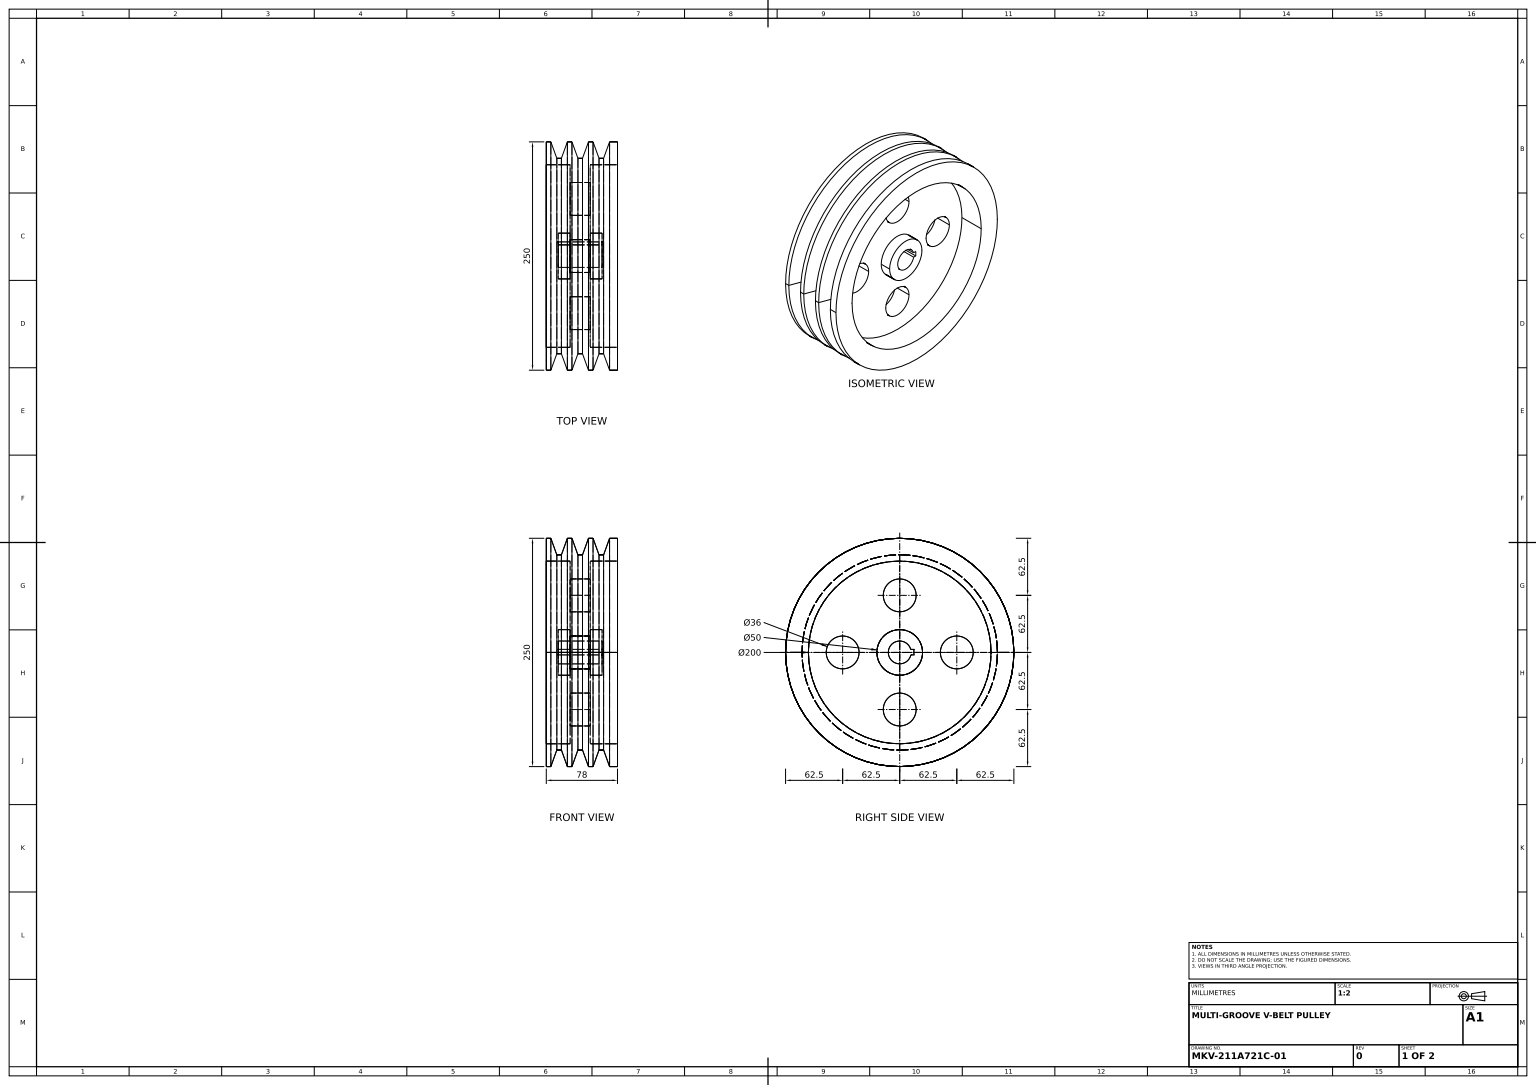
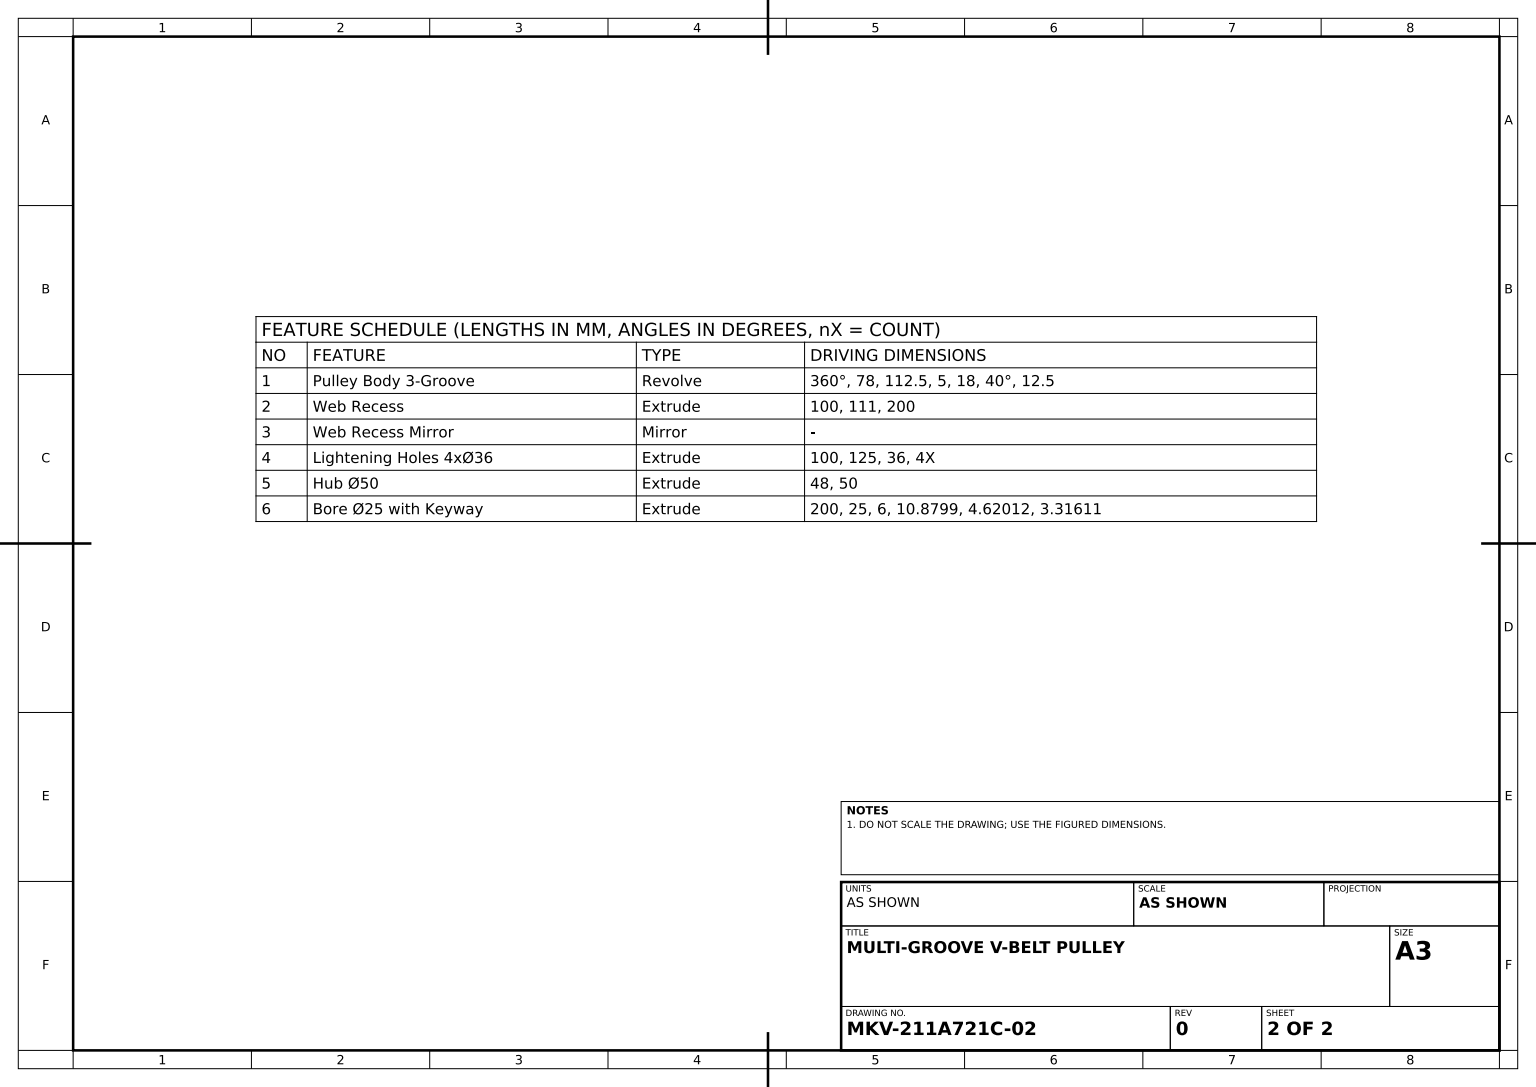
from build123d import *

# Parameters (mm, degrees)
WEB_START                    = 111
WEB_RECESS_SKETCH_R          = 100
WEB_RECESS_DEPTH             = 100
LIGHTENING_HOLES_SKETCH_R    = 18
LIGHTENING_HOLES_4X_36_DEPTH = 50
HUB_SKETCH_R                 = 25
HUB_50_DEPTH                 = 24
BORE_KEYWAY_SKETCH_R         = 12.5
BORE_KEYWAY_SKETCH_W         = 10.879881684
BORE_KEYWAY_SKETCH_H         = 6
BORE_25_WITH_KEYWAY_DEPTH    = 100


with BuildPart() as part:
    # Pulley Profile Sketch → Pulley Body 3-Groove (revolve)
    with BuildSketch(Plane.XY, mode=Mode.PRIVATE) as pulley_body_3_groove_sk:
        Polygon((-2.5, 107), (2.5, 107), (9.051464217, 125), (14.051464217, 125), (20.602928434, 107), (25.602928434, 107), (32.15439265, 125), (40.84560735, 125), (40.84560735, 12.5), (-37.15439265, 12.5), (-37.15439265, 125), (-32.15439265, 125), (-25.602928434, 107), (-20.602928434, 107), (-14.051464217, 125), (-9.051464217, 125), align=None)
    revolve(pulley_body_3_groove_sk.sketch.rotate(Axis((491.806779687, 0, 0), (-1, 0, 0)), 90), axis=Axis((491.806779687, 0, 0), (-1, 0, 0)))

    # Web Recess Sketch → Web Recess (cut)
    with BuildSketch(Plane(origin=(0, 0, 0), x_dir=(0, 0, -1), z_dir=(1, 0, 0)).offset(WEB_START)):
        Circle(WEB_RECESS_SKETCH_R)
    web_recess = extrude(amount=-WEB_RECESS_DEPTH, mode=Mode.SUBTRACT)

    # Web Recess Mirror: Web Recess across plane
    add(web_recess.mirror(Plane(origin=(0, 0, 0), x_dir=(0, 0, 1), z_dir=(1, 0, 0))), mode=Mode.SUBTRACT)

    # Lightening Holes Sketch → Lightening Holes 4xØ36 (cut, symmetric)
    with BuildSketch(Plane(origin=(0, 0, 0), x_dir=(0, 0, -1), z_dir=(1, 0, 0))):
        with Locations((62.5, 0)):
            Circle(LIGHTENING_HOLES_SKETCH_R)
        with Locations((0, -62.5)):
            Circle(LIGHTENING_HOLES_SKETCH_R)
        with Locations((-62.5, 0)):
            Circle(LIGHTENING_HOLES_SKETCH_R)
        with Locations((0, 62.5)):
            Circle(LIGHTENING_HOLES_SKETCH_R)
    extrude(amount=LIGHTENING_HOLES_4X_36_DEPTH, both=True, mode=Mode.SUBTRACT)

    # Hub Sketch → Hub Ø50 (add, symmetric)
    with BuildSketch(Plane(origin=(0, 0, 0), x_dir=(0, 0, -1), z_dir=(1, 0, 0))):
        with Locations(Location((0, 0, 0), (0, 0, 180))):
            Circle(HUB_SKETCH_R)
    extrude(amount=HUB_50_DEPTH, both=True)

    # Bore Keyway Sketch → Bore Ø25 with Keyway (cut, symmetric)
    with BuildSketch(Plane(origin=(0, 0, 0), x_dir=(0, 0, -1), z_dir=(1, 0, 0))):
        Circle(BORE_KEYWAY_SKETCH_R)
        with Locations((10.060059158, 0.316113857)):
            Rectangle(BORE_KEYWAY_SKETCH_W, BORE_KEYWAY_SKETCH_H)
    extrude(amount=BORE_25_WITH_KEYWAY_DEPTH, both=True, mode=Mode.SUBTRACT)


solid = part.part
